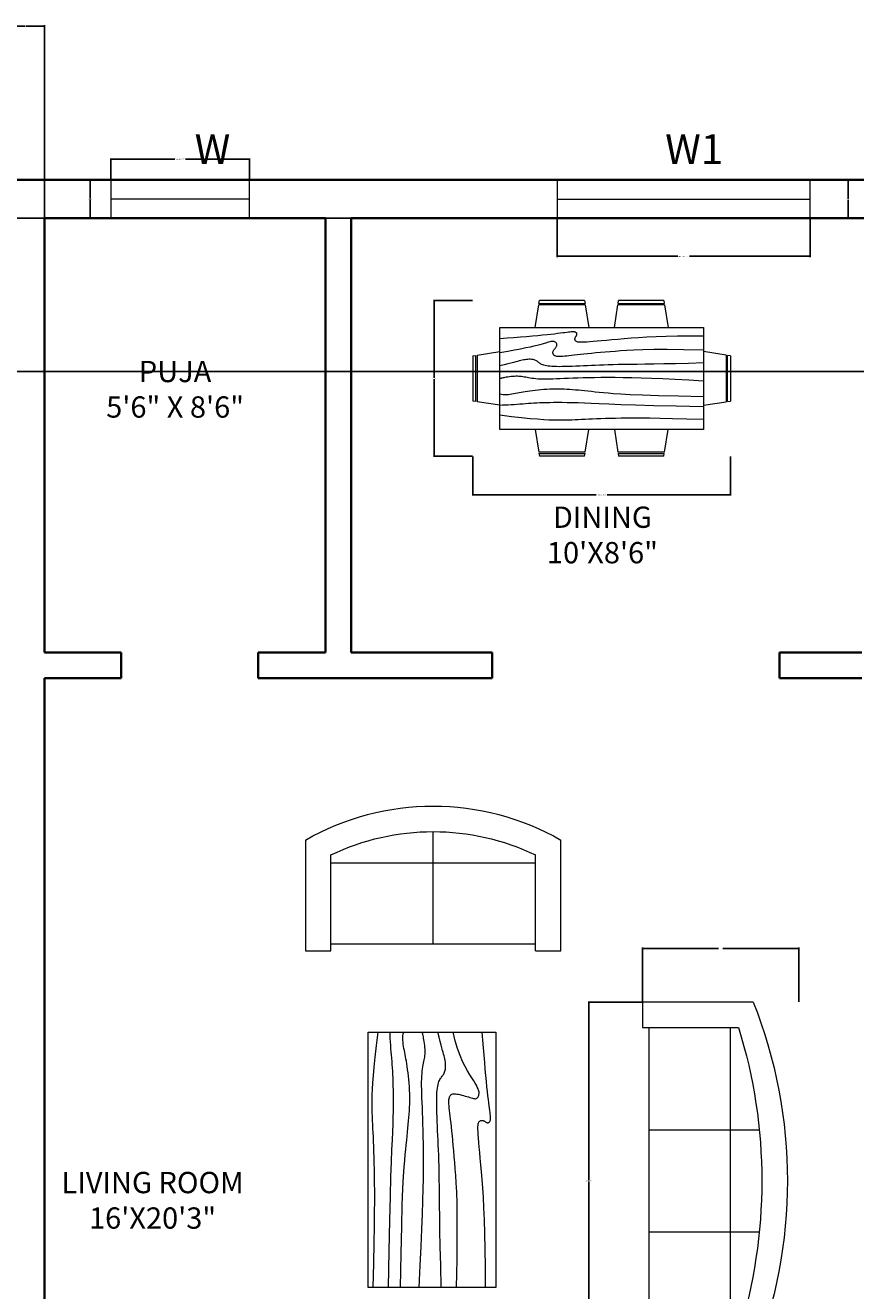
# Model space of a CAD drawing. Units: inches. Extents: x 1939 to 2674, y 558 to 1170.
# Tile 5 of 6: x 2307 to 2502, y 873 to 1170. Entities that reach past the tile are written whole.
import ezdxf

# ---------------------------------------------------------------- set-up
doc = ezdxf.new("R2010")
doc.units = ezdxf.units.IN
for name, color, linetype, lineweight in [('A-ANNO-DIMS', 2, 'Continuous', 18), ('A-ANNO-TEXT', 7, 'Continuous', 18), ('A-AREA-IDEN', 7, 'Continuous', 18), ('A-FURN', 8, 'Continuous', 13), ('A-GLAZ', 4, 'Continuous', 18), ('A-WALL', 7, 'Continuous', 35)]:
    doc.layers.add(name, color=color, linetype=linetype, lineweight=lineweight)
doc.styles.get("Standard").update_dxf_attribs({"font": 'arial.ttf'})
doc.dimstyles.get("Standard").update_dxf_attribs({"dimtxt": 0.18, "dimasz": 0.18, "dimexe": 0.18, "dimexo": 0.0625, "dimgap": 0.09, "dimtad": 0, "dimtih": 1, "dimtoh": 1, "dimdec": 4, "dimzin": 0, "dimdsep": 46, "dimtxsty": 'Standard', "dimcen": 0.09, "dimadec": 0, "dimazin": 0, "dimtfac": 1, "dimtdec": 4, "dimtofl": 0, "dimtmove": 0, "dimatfit": 3, "dimfxl": 1, "dimtolj": 1, "dimtzin": 0, "dimarcsym": 0})

# ---------------------------------------------------------------- blocks, each defined once
blk = doc.blocks.new('Dining Set - 36 x 72 in.')
for p, q in [((-22, 27.5), (-22.1562, 26.50042)), ((-22, 27.5), (-6, 27.5)), ((-5.8437, 26.49966), (-6, 27.5)), ((6, 27.5), (5.8438, 26.50042)), ((6, 27.5), (22, 27.5)), ((22.1563, 26.49966), (22, 27.5)), ((-22.2343, 26.00059), (-23.4847, 17.99762)), ((-22.2304, 26), (-5.7608, 26)), ((-5.8416, 26.5), (-22.1534, 26.5)), ((-4.5152, 17.99762), (-5.7655, 25.99926)), ((5.7657, 26.00059), (4.5153, 17.99762)), ((5.7696, 26), (22.2392, 26)), ((22.1584, 26.5), (5.8466, 26.5)), ((23.4848, 17.99762), (22.2345, 25.99926)), ((36, 18), (-36, 18)), ((-36, 18), (-36, -18)), ((36, -18), (36, 18)), ((-44.0006, 8.23428), (-35.9976, 9.48474)), ((44.0006, 8.23428), (35.9976, 9.48474)), ((-45.5, 8), (-44.5004, 8.15617)), ((-45.5, 8), (-45.5, -8)), ((-44.5, -8.15843), (-44.5, 8.15338)), ((-44, 8.23041), (-44, -8.23915)), ((44, 8.23041), (44, -8.23915)), ((44.5, -8.15843), (44.5, 8.15338)), ((45.5, 8), (44.5005, 8.15617)), ((45.5, 8), (45.5, -8)), ((-44.4997, -8.15631), (-45.5, -8)), ((-35.9976, -9.48476), (-43.9993, -8.2345)), ((35.9976, -9.48476), (43.9993, -8.2345)), ((44.4997, -8.15631), (45.5, -8)), ((-36, -18), (36, -18)), ((-22.2343, -26.0006), (-23.4847, -17.99762)), ((-4.5152, -17.99762), (-5.7655, -25.99928)), ((5.7657, -26.0006), (4.5153, -17.99762)), ((23.4848, -17.99762), (22.2345, -25.99928)), ((-22.2304, -26), (-5.7608, -26)), ((-22, -27.5), (-22.1562, -26.50044)), ((-5.8416, -26.5), (-22.1534, -26.5)), ((-5.8437, -26.49967), (-6, -27.5)), ((5.7696, -26), (22.2392, -26)), ((6, -27.5), (5.8438, -26.50044)), ((22.1584, -26.5), (5.8466, -26.5)), ((22.1563, -26.49967), (22, -27.5)), ((-22, -27.5), (-6, -27.5)), ((6, -27.5), (22, -27.5))]:
    blk.add_line(p, q)
for points in [[(-36, 15), (-31.1772, 14.97754), (-26.8079, 14.91406), (-22.8538, 14.81543), (-19.276, 14.6875), (-16.0362, 14.53613), (-13.0957, 14.36718), (-10.4159, 14.18652), (-7.9583, 14), (-5.6904, 13.81315), (-3.6035, 13.63021), (-1.6954, 13.45508), (0.0365, 13.29166), (1.5945, 13.14388), (2.9811, 13.01562), (4.1988, 12.9108), (5.25, 12.83333), (6.1393, 12.78613), (6.8802, 12.76823), (7.4883, 12.77767), (7.9792, 12.8125), (8.3685, 12.87077), (8.6719, 12.95052), (8.9049, 13.0498), (9.0833, 13.16666), (9.2205, 13.29899), (9.3216, 13.44401), (9.3895, 13.59879), (9.4271, 13.76041), (9.4373, 13.92594), (9.4232, 14.09245), (9.3875, 14.257), (9.3333, 14.41666), (9.2638, 14.56917), (9.1836, 14.71484), (9.0975, 14.85465), (9.0104, 14.98958), (8.9272, 15.1206), (8.8529, 15.2487), (8.7922, 15.37483), (8.75, 15.5), (8.7305, 15.62467), (8.7344, 15.74739), (8.7617, 15.86621), (8.8125, 15.97916), (8.8867, 16.08431), (8.9844, 16.17968), (9.1055, 16.26334), (9.25, 16.33333), (9.4189, 16.38802), (9.6172, 16.42708), (9.8506, 16.45052), (10.125, 16.45833), (10.4463, 16.45052), (10.8203, 16.42708), (11.2529, 16.38802), (11.75, 16.33333), (12.3184, 16.26318), (12.9694, 16.17838), (13.7151, 16.07991), (14.5677, 15.96875), (15.5395, 15.84586), (16.6426, 15.71224), (17.8893, 15.56884), (19.2917, 15.41666), (20.859, 15.25667), (22.5879, 15.08984), (24.4721, 14.91715), (26.5052, 14.73958), (28.6809, 14.5581), (30.9929, 14.3737), (33.4347, 14.18733), (36, 14)], [(-36, 10), (-28.9766, 10.14274), (-23.1725, 10.20442), (-18.4241, 10.19775), (-14.5677, 10.13541), (-11.4399, 10.03011), (-8.877, 9.89453), (-6.7154, 9.74137), (-4.7917, 9.58333), (-2.9698, 9.43082), (-1.2246, 9.28515), (0.4415, 9.14534), (2.026, 9.01041), (3.5266, 8.87939), (4.9408, 8.7513), (6.266, 8.62516), (7.5, 8.5), (8.6411, 8.37549), (9.6914, 8.2539), (10.6538, 8.13818), (11.5312, 8.03125), (12.3267, 7.93603), (13.043, 7.85547), (13.6831, 7.79248), (14.25, 7.75), (14.7471, 7.7303), (15.1797, 7.73307), (15.5537, 7.75732), (15.875, 7.80208), (16.1494, 7.86637), (16.3828, 7.94922), (16.5811, 8.04964), (16.75, 8.16666), (16.8944, 8.29915), (17.0143, 8.44531), (17.1089, 8.60319), (17.1771, 8.77083), (17.218, 8.94629), (17.2305, 9.1276), (17.2137, 9.31282), (17.1667, 9.5), (17.0895, 9.6875), (16.987, 9.875), (16.8649, 10.0625), (16.7292, 10.25), (16.5856, 10.4375), (16.4401, 10.625), (16.2985, 10.8125), (16.1667, 11), (16.05, 11.18733), (15.9518, 11.3737), (15.8752, 11.5581), (15.8229, 11.73958), (15.798, 11.91715), (15.8034, 12.08984), (15.842, 12.25667), (15.9167, 12.41666), (16.0295, 12.56836), (16.1784, 12.70833), (16.3605, 12.83268), (16.5729, 12.9375), (16.8127, 13.01888), (17.0768, 13.07291), (17.3625, 13.0957), (17.6667, 13.08333), (17.9894, 13.03312), (18.3418, 12.94726), (18.7382, 12.82918), (19.1927, 12.68229), (19.7195, 12.51001), (20.3327, 12.31575), (21.0465, 12.10294), (21.875, 11.875), (22.8357, 11.63354), (23.959, 11.37304), (25.2786, 11.08618), (26.8282, 10.76562), (28.6414, 10.40405), (30.752, 9.99414), (33.1936, 9.52856), (36, 9)], [(-36, 5.5), (-30.7157, 5.3348), (-26.069, 5.20963), (-21.9946, 5.11767), (-18.4271, 5.05208), (-15.3009, 5.00602), (-12.5508, 4.97265), (-10.1112, 4.94515), (-7.9167, 4.91666), (-5.909, 4.88167), (-4.0586, 4.83984), (-2.3429, 4.79215), (-0.7396, 4.73958), (0.7739, 4.6831), (2.22, 4.6237), (3.6213, 4.56233), (5, 4.5), (6.373, 4.43782), (7.7344, 4.3776), (9.0723, 4.32129), (10.375, 4.27083), (11.6309, 4.22819), (12.8281, 4.19531), (13.9551, 4.17415), (15, 4.16666), (15.954, 4.17448), (16.819, 4.19791), (17.6001, 4.23698), (18.3021, 4.29166), (18.9299, 4.36198), (19.4883, 4.44791), (19.9823, 4.54948), (20.4167, 4.66666), (20.7969, 4.79899), (21.1302, 4.94401), (21.4245, 5.09879), (21.6875, 5.26041), (21.9271, 5.42594), (22.1511, 5.59245), (22.3672, 5.757), (22.5834, 5.91666), (22.8065, 6.06868), (23.0404, 6.21093), (23.2879, 6.34147), (23.5521, 6.45833), (23.8358, 6.55957), (24.142, 6.64323), (24.4735, 6.70735), (24.8334, 6.75), (25.2235, 6.76969), (25.642, 6.76692), (26.0858, 6.74267), (26.5521, 6.69791), (27.0379, 6.63362), (27.5404, 6.55078), (28.0565, 6.45036), (28.5834, 6.33333), (29.1242, 6.19987), (29.7071, 6.04687), (30.3661, 5.87044), (31.1354, 5.66666), (32.0493, 5.43164), (33.142, 5.16146), (34.4475, 4.85221), (36, 4.5)], [(-36, -1), (-30.7915, -0.6591), (-26.0195, -0.38216), (-21.6519, -0.16284), (-17.6563, 0.00521), (-14.0005, 0.12833), (-10.6523, 0.21289), (-7.5796, 0.26522), (-4.75, 0.29166), (-2.134, 0.29793), (0.2878, 0.28711), (2.5317, 0.26163), (4.6146, 0.22396), (6.5529, 0.17651), (8.3633, 0.12174), (10.0623, 0.06209), (11.6667, 0), (13.1899, -0.06201), (14.6341, -0.1211), (15.9982, -0.17432), (17.2813, -0.21875), (18.4823, -0.25147), (19.6003, -0.26953), (20.6343, -0.27002), (21.5834, -0.25), (22.4481, -0.20768), (23.2357, -0.14584), (23.9549, -0.06836), (24.6146, 0.02083), (25.2235, 0.11784), (25.7904, 0.21875), (26.3241, 0.31966), (26.8334, 0.41666), (27.3265, 0.50618), (27.8099, 0.58593), (28.2894, 0.65397), (28.7709, 0.70833), (29.2601, 0.74707), (29.763, 0.76823), (30.2855, 0.76985), (30.8334, 0.75), (31.4088, 0.70784), (31.9994, 0.64713), (32.589, 0.57275), (33.1615, 0.48958), (33.7008, 0.4025), (34.1908, 0.3164), (34.6153, 0.23616), (34.9584, 0.16666), (35.2099, 0.11165), (35.3848, 0.07031), (35.504, 0.04069), (35.5886, 0.02083), (35.6594, 0.00879), (35.7377, 0.0026), (35.8442, 0.00032), (36, 0)], [(-36, -6.5), (-27.1843, -6.31267), (-20.084, -6.1263), (-14.469, -5.9419), (-10.1094, -5.76042), (-6.7752, -5.58285), (-4.2363, -5.41016), (-2.2629, -5.24333), (-0.625, -5.08334), (0.8708, -4.93099), (2.2715, -4.78646), (3.5872, -4.64974), (4.8281, -4.52084), (6.0046, -4.39974), (7.127, -4.28646), (8.2053, -4.18099), (9.25, -4.08334), (10.2705, -3.99382), (11.2734, -3.91407), (12.2647, -3.84603), (13.25, -3.79167), (14.2354, -3.75293), (15.2266, -3.73177), (16.2295, -3.73015), (17.25, -3.75), (18.2912, -3.79248), (19.3451, -3.85547), (20.4009, -3.93604), (21.4479, -4.03125), (22.4754, -4.13819), (23.4727, -4.25391), (24.4289, -4.37549), (25.3334, -4.5), (26.1785, -4.62492), (26.9694, -4.74935), (27.7145, -4.87281), (28.4219, -4.99479), (29.1, -5.11483), (29.7572, -5.23242), (30.4016, -5.34709), (31.0417, -5.45834), (31.6837, -5.56437), (32.3262, -5.65821), (32.9658, -5.73153), (33.599, -5.77604), (34.2224, -5.78345), (34.8327, -5.74545), (35.4264, -5.65373), (36, -5.5)], [(-36, -10), (-26.4022, -9.81299), (-18.4675, -9.62891), (-11.9839, -9.45069), (-6.7396, -9.28125), (-2.5226, -9.12354), (0.8789, -8.98047), (3.6769, -8.85498), (6.0833, -8.75), (8.2767, -8.66765), (10.3021, -8.60677), (12.1712, -8.56543), (13.8958, -8.54167), (15.4876, -8.53353), (16.9583, -8.53907), (18.3197, -8.55632), (19.5834, -8.58334), (20.7616, -8.61841), (21.8685, -8.66081), (22.9188, -8.71004), (23.9271, -8.76563), (24.9081, -8.82707), (25.8763, -8.89388), (26.8465, -8.96558), (27.8334, -9.04167), (28.8474, -9.12118), (29.8828, -9.20117), (30.93, -9.27824), (31.9792, -9.34896), (33.0205, -9.40991), (34.0443, -9.45768), (35.0407, -9.48885), (36, -9.5)], [(-36, -14.5), (-30.0881, -14.33513), (-25.0332, -14.21224), (-20.7312, -14.12647), (-17.0781, -14.07292), (-13.97, -14.04671), (-11.3027, -14.04297), (-8.9724, -14.05681), (-6.875, -14.08334), (-4.9224, -14.11833), (-3.0905, -14.16016), (-1.3709, -14.20785), (0.2448, -14.26042), (1.7647, -14.3169), (3.1973, -14.3763), (4.5507, -14.43767), (5.8333, -14.5), (7.0554, -14.5621), (8.235, -14.62175), (9.3922, -14.67652), (10.5469, -14.72396), (11.7192, -14.76164), (12.929, -14.78711), (14.1965, -14.79794), (15.5417, -14.79167), (16.9933, -14.76424), (18.6152, -14.70508), (20.4804, -14.60197), (22.6615, -14.44271), (25.2312, -14.21509), (28.2624, -13.9069), (31.8277, -13.50594), (36, -13)]]:
    blk.add_lwpolyline(points)
blk = doc.blocks.new('Sofa - Roundback 7 ft.')
for p, q in [((-12.00002, -32.4421), (-12.00003, -6.5971)), ((11.99997, -32.4421), (11.99998, -6.5971)), ((-36.000027, -34), (-36.000027, -11.4696)), ((35.99998, -34), (35.99998, -11.4696)), ((-35.999844, -13.3819), (35.9998, -13.3819)), ((-36.000027, -32.4421), (35.99998, -32.4421))]:
    blk.add_line(p, q)
for points in [[(-36.000027, -34), (-42.000027, -34), (-42.000027, -8)], [(41.99998, -8), (41.99998, -34), (35.99998, -34)]]:
    blk.add_lwpolyline(points)
for centre, radius, start, end in [((0, -114.25), 114.25, 68.43141, 111.5686), ((-0.00001, -127.1968), 121.1968, 72.72033, 107.2797)]:
    blk.add_arc(centre, radius, start, end)
blk = doc.blocks.new('Sofa - Roundback Loveseat 5 ft.')
for p, q in [((0, -32.44198), (0, -5.99998)), ((-24, -33.99998), (-24, -11.46958)), ((24.00004, -33.99998), (24.00004, -11.46958)), ((-23.9998, -13.38178), (23.99986, -13.38178)), ((-24, -32.44198), (24.00004, -32.44198))]:
    blk.add_line(p, q)
for points in [[(-24, -33.99998), (-30, -33.99998), (-30, -7.99998)], [(30.00004, -7.99998), (30.00004, -33.99998), (24.00004, -33.99998)]]:
    blk.add_lwpolyline(points)
for centre, radius, start, end in [((0, -60.24998), 60.24998, 60.13715, 119.8628), ((0, -61.38438), 55.38444, 64.32083, 115.6792)]:
    blk.add_arc(centre, radius, start, end)
blk = doc.blocks.new('Table - Rectangular Woodgrain 60 x 30 in.')
for p, q in [((0, 0), (0, -30)), ((60, 0), (0, 0)), ((60, -30), (60, 0)), ((0, -30), (60, -30))]:
    blk.add_line(p, q)
for points in [[(0, -2.4), (4.8155, -2.418), (9.0302, -2.4688), (12.709, -2.5477), (15.9167, -2.65), (18.7181, -2.7711), (21.1781, -2.9063), (23.3616, -3.0508), (25.3333, -3.2), (27.1477, -3.3495), (28.8172, -3.4958), (30.3437, -3.636), (31.7291, -3.7667), (32.9756, -3.8849), (34.0849, -3.9875), (35.059, -4.0714), (35.9, -4.1334), (36.6114, -4.1711), (37.2041, -4.1854), (37.6906, -4.1779), (38.0833, -4.15), (38.3948, -4.1034), (38.6375, -4.0396), (38.8239, -3.9602), (38.9666, -3.8667), (39.0764, -3.7608), (39.1573, -3.6448), (39.2116, -3.521), (39.2416, -3.3917), (39.2498, -3.2593), (39.2385, -3.1261), (39.21, -2.9944), (39.1666, -2.8667), (39.111, -2.7447), (39.0468, -2.6281), (38.978, -2.5163), (38.9083, -2.4083), (38.8418, -2.3035), (38.7823, -2.201), (38.7337, -2.1001), (38.7, -2), (38.6844, -1.9003), (38.6875, -1.8021), (38.7094, -1.707), (38.75, -1.6167), (38.8094, -1.5326), (38.8875, -1.4563), (38.9844, -1.3893), (39.1, -1.3333), (39.2351, -1.2896), (39.3937, -1.2583), (39.5804, -1.2396), (39.8, -1.2333), (40.057, -1.2396), (40.3562, -1.2583), (40.7023, -1.2896), (41.1, -1.3333), (41.5547, -1.3895), (42.0755, -1.4573), (42.6721, -1.5361), (43.3542, -1.625), (44.1316, -1.7233), (45.014, -1.8302), (46.0114, -1.9449), (47.1333, -2.0667), (48.3862, -2.1947), (49.7625, -2.3281), (51.2513, -2.4663), (52.8416, -2.6083), (54.5226, -2.7535), (56.2833, -2.9011), (58.1127, -3.0501), (60, -3.2)], [(0, -9.2), (6.5759, -9.0858), (11.9385, -9.0365), (16.2527, -9.0418), (19.6833, -9.0917), (22.3952, -9.1759), (24.5531, -9.2844), (26.322, -9.4069), (27.8666, -9.5333), (29.3241, -9.6553), (30.7203, -9.7719), (32.0532, -9.8837), (33.3208, -9.9917), (34.5213, -10.0965), (35.6526, -10.199), (36.7128, -10.2999), (37.7, -10.4), (38.6129, -10.4996), (39.4531, -10.5969), (40.223, -10.6895), (40.925, -10.775), (41.5613, -10.8512), (42.1344, -10.9156), (42.6465, -10.966), (43.1, -11), (43.4976, -11.0158), (43.8437, -11.0136), (44.143, -10.9942), (44.4, -10.9583), (44.6195, -10.9069), (44.8062, -10.8406), (44.9648, -10.7603), (45.1, -10.6667), (45.2155, -10.5598), (45.3114, -10.4365), (45.3871, -10.2929), (45.4416, -10.125), (45.4743, -9.929), (45.4844, -9.7011), (45.4709, -9.4371), (45.4333, -9.1333), (45.3716, -8.7883), (45.2896, -8.4104), (45.1919, -8.0107), (45.0833, -7.6), (44.9685, -7.1893), (44.8521, -6.7896), (44.7388, -6.4117), (44.6333, -6.0667), (44.54, -5.7628), (44.4614, -5.4979), (44.4001, -5.2675), (44.3583, -5.0667), (44.3384, -4.8909), (44.3427, -4.7354), (44.3736, -4.5956), (44.4333, -4.4667), (44.5236, -4.3453), (44.6427, -4.2333), (44.7884, -4.1339), (44.9583, -4.05), (45.1501, -3.9849), (45.3614, -3.9417), (45.59, -3.9234), (45.8333, -3.9333), (46.0915, -3.9749), (46.3734, -4.0531), (46.6906, -4.1736), (47.0542, -4.3417), (47.4756, -4.5629), (47.9661, -4.8427), (48.5372, -5.1866), (49.2, -5.6), (49.9676, -6.0844), (50.8594, -6.625), (51.8965, -7.2031), (53.1, -7.8), (54.491, -8.3969), (56.0906, -8.975), (57.9199, -9.5156), (60, -10)], [(0, -12.8), (5.1847, -12.9322), (9.6213, -13.0323), (13.3963, -13.1059), (16.5958, -13.1583), (19.3063, -13.1952), (21.614, -13.2219), (23.6054, -13.2439), (25.3666, -13.2667), (26.9728, -13.2947), (28.4531, -13.3281), (29.8256, -13.3663), (31.1083, -13.4083), (32.3191, -13.4535), (33.476, -13.501), (34.597, -13.5501), (35.7, -13.6), (36.7984, -13.6497), (37.8875, -13.6979), (38.9578, -13.743), (40, -13.7833), (41.0047, -13.8174), (41.9625, -13.8438), (42.864, -13.8607), (43.7, -13.8667), (44.4631, -13.8604), (45.1552, -13.8417), (45.7801, -13.8104), (46.3416, -13.7667), (46.8439, -13.7104), (47.2906, -13.6417), (47.6858, -13.5604), (48.0333, -13.4667), (48.3375, -13.3608), (48.6042, -13.2448), (48.8396, -13.121), (49.05, -12.9917), (49.2417, -12.8593), (49.4208, -12.7261), (49.5937, -12.5944), (49.7667, -12.4667), (49.9452, -12.3451), (50.1323, -12.2313), (50.3303, -12.1268), (50.5416, -12.0333), (50.7686, -11.9524), (51.0135, -11.8854), (51.2788, -11.8341), (51.5666, -11.8), (51.8785, -11.7843), (52.2116, -11.7865), (52.562, -11.8059), (52.926, -11.8417), (53.2998, -11.8931), (53.6795, -11.9594), (54.0614, -12.0397), (54.4416, -12.1333), (54.8223, -12.2401), (55.2293, -12.3625), (55.6942, -12.5037), (56.2489, -12.6667), (56.9251, -12.8547), (57.7545, -13.0708), (58.7689, -13.3182), (60, -13.6)], [(0, -18), (5.124, -17.7273), (9.6609, -17.5057), (13.6705, -17.3303), (17.2125, -17.1958), (20.3467, -17.0973), (23.1328, -17.0297), (25.6307, -16.9878), (27.9, -16.9667), (29.9928, -16.9617), (31.9302, -16.9703), (33.7254, -16.9907), (35.3917, -17.0208), (36.9423, -17.0588), (38.3906, -17.1026), (39.7499, -17.1503), (41.0333, -17.2), (42.2519, -17.2496), (43.4073, -17.2969), (44.4986, -17.3395), (45.525, -17.375), (46.4858, -17.4012), (47.3802, -17.4156), (48.2074, -17.416), (48.9667, -17.4), (49.6583, -17.3662), (50.2872, -17.3167), (50.8595, -17.2547), (51.3812, -17.1833), (51.8584, -17.1057), (52.2971, -17.025), (52.7034, -16.9443), (53.0833, -16.8667), (53.443, -16.7951), (53.789, -16.7313), (54.128, -16.6768), (54.4666, -16.6334), (54.8115, -16.6024), (55.1693, -16.5854), (55.5465, -16.5841), (55.95, -16.6), (56.3828, -16.6337), (56.8346, -16.6823), (57.2915, -16.7418), (57.7396, -16.8084), (58.165, -16.878), (58.5539, -16.9469), (58.8924, -17.0111), (59.1666, -17.0667), (59.3679, -17.1107), (59.5078, -17.1438), (59.6032, -17.1675), (59.6708, -17.1833), (59.7275, -17.193), (59.7901, -17.1979), (59.8753, -17.1998), (60, -17.2)], [(0, -22.4), (8.0098, -22.2501), (14.4094, -22.1011), (19.4168, -21.9535), (23.25, -21.8083), (26.1269, -21.6663), (28.2656, -21.5281), (29.884, -21.3947), (31.2, -21.2667), (32.3967, -21.1448), (33.5172, -21.0292), (34.5697, -20.9198), (35.5625, -20.8167), (36.5037, -20.7198), (37.4015, -20.6292), (38.2642, -20.5448), (39.1, -20.4667), (39.9164, -20.3951), (40.7187, -20.3313), (41.5117, -20.2768), (42.3, -20.2333), (43.0883, -20.2024), (43.8812, -20.1854), (44.6836, -20.1841), (45.5, -20.2), (46.3328, -20.234), (47.1747, -20.2844), (48.0163, -20.3488), (48.8479, -20.425), (49.66, -20.5106), (50.4429, -20.6031), (51.1872, -20.7004), (51.8833, -20.8), (52.5246, -20.8999), (53.1166, -20.9995), (53.6681, -21.0983), (54.1875, -21.1958), (54.6834, -21.2919), (55.1646, -21.3859), (55.6394, -21.4777), (56.1167, -21.5667), (56.6028, -21.6515), (57.0961, -21.7266), (57.5929, -21.7852), (58.0896, -21.8208), (58.5823, -21.8268), (59.0674, -21.7964), (59.5412, -21.723), (60, -21.6)], [(0, -25.2), (8.6355, -25.0504), (15.7026, -24.9031), (21.4049, -24.7606), (25.9458, -24.625), (29.529, -24.4988), (32.3578, -24.3844), (34.6359, -24.284), (36.5667, -24.2), (38.3213, -24.1341), (39.9417, -24.0854), (41.437, -24.0523), (42.8167, -24.0333), (44.0901, -24.0268), (45.2667, -24.0313), (46.3557, -24.0451), (47.3667, -24.0667), (48.309, -24.0947), (49.1928, -24.1287), (50.0284, -24.168), (50.826, -24.2125), (51.5959, -24.2617), (52.3483, -24.3151), (53.0935, -24.3725), (53.8417, -24.4334), (54.6009, -24.497), (55.3699, -24.561), (56.1454, -24.6226), (56.9239, -24.6792), (57.7021, -24.7279), (58.4764, -24.7662), (59.2435, -24.7911), (60, -24.8)], [(0, -28.8), (5.6867, -28.6681), (10.45, -28.5698), (14.407, -28.5012), (17.675, -28.4584), (20.3711, -28.4374), (22.6125, -28.4344), (24.5164, -28.4455), (26.2, -28.4667), (27.762, -28.4947), (29.2276, -28.5281), (30.6033, -28.5663), (31.8958, -28.6084), (33.1118, -28.6535), (34.2578, -28.7011), (35.3405, -28.7501), (36.3666, -28.8), (37.3443, -28.8497), (38.288, -28.8974), (39.2137, -28.9412), (40.1375, -28.9792), (41.0753, -29.0093), (42.0432, -29.0297), (43.0572, -29.0384), (44.1333, -29.0333), (45.2936, -29.0114), (46.5843, -28.9641), (48.0579, -28.8816), (49.7666, -28.7542), (51.7629, -28.5721), (54.0989, -28.3255), (56.8272, -28.0048), (60, -27.6)]]:
    blk.add_lwpolyline(points)
blk = doc.blocks.new('WIN-PUJA')
for p, q in [((0, 9), (0, 0)), ((32.53, 0), (32.53, 9)), ((0, 4.5), (32.53, 4.5))]:
    blk.add_line(p, q)
blk = doc.blocks.new('WIN-DINING')
for p, q in [((0, 9), (0, 0)), ((59.38, 0), (59.38, 9)), ((0, 4.5), (59.38, 4.5))]:
    blk.add_line(p, q)
blk = doc.blocks.new('*D24')
at = {"layer": 'A-ANNO-DIMS', "color": 0, "lineweight": -2, "transparency": 16777216}
for p, q in [((2411.67, 1069.16), (2411.67, 1059.97)), ((2472.14, 1069.16), (2472.14, 1059.97)), ((2411.85, 1060.15), (2440.62, 1060.15)), ((2471.96, 1060.15), (2443.18, 1060.15))]:
    blk.add_line(p, q, dxfattribs=at)
at = {"layer": 'A-ANNO-DIMS', "color": 0, "transparency": 16777216}
for points in [[(2411.85, 1060.18), (2411.85, 1060.12), (2411.67, 1060.15)], [(2471.96, 1060.18), (2471.96, 1060.12), (2472.14, 1060.15)]]:
    blk.add_solid(points, dxfattribs=at)
at = {"layer": 'Defpoints', "color": 0, "transparency": 16777216}
for p in [(2411.67, 1069.22), (2472.14, 1069.22), (2411.67, 1060.15)]:
    blk.add_point(p, dxfattribs=at)
at = {"layer": 'A-ANNO-DIMS', "color": 0, "transparency": 16777216, "insert": (2441.9, 1060.15), "char_height": 0.18, "attachment_point": 5}
blk.add_mtext('\\A1;DINING SET 60 TYP.', dxfattribs=at)
blk = doc.blocks.new('*D25')
at = {"layer": 'A-ANNO-DIMS', "color": 0, "lineweight": -2, "transparency": 16777216}
for p, q in [((2411.61, 1105.77), (2402.42, 1105.77)), ((2402.6, 1105.59), (2402.6, 1087.68)), ((2402.6, 1069.4), (2402.6, 1087.32)), ((2411.61, 1069.22), (2402.42, 1069.22))]:
    blk.add_line(p, q, dxfattribs=at)
at = {"layer": 'A-ANNO-DIMS', "color": 0, "transparency": 16777216}
for points in [[(2402.57, 1105.59), (2402.63, 1105.59), (2402.6, 1105.77)], [(2402.57, 1069.4), (2402.63, 1069.4), (2402.6, 1069.22)]]:
    blk.add_solid(points, dxfattribs=at)
at = {"layer": 'Defpoints', "color": 0, "transparency": 16777216}
for p in [(2402.6, 1105.77), (2411.67, 1105.77), (2411.67, 1069.22)]:
    blk.add_point(p, dxfattribs=at)
at = {"layer": 'A-ANNO-DIMS', "color": 0, "transparency": 16777216, "insert": (2402.6, 1087.5), "char_height": 0.18, "attachment_point": 5}
blk.add_mtext('\\A1;37 TYP.', dxfattribs=at)
blk = doc.blocks.new('*D26')
at = {"layer": 'A-ANNO-DIMS', "color": 0, "lineweight": -2, "transparency": 16777216}
for p, q in [((2451.46, 941.04), (2438.74, 941.04)), ((2438.92, 940.86), (2438.92, 899.23)), ((2438.92, 857.22), (2438.92, 898.86)), ((2451.46, 857.04), (2438.74, 857.04))]:
    blk.add_line(p, q, dxfattribs=at)
at = {"layer": 'A-ANNO-DIMS', "color": 0, "transparency": 16777216}
for points in [[(2438.89, 940.86), (2438.95, 940.86), (2438.92, 941.04)], [(2438.89, 857.22), (2438.95, 857.22), (2438.92, 857.04)]]:
    blk.add_solid(points, dxfattribs=at)
at = {"layer": 'Defpoints', "color": 0, "transparency": 16777216}
for p in [(2438.92, 941.04), (2451.52, 941.04), (2451.52, 857.04)]:
    blk.add_point(p, dxfattribs=at)
at = {"layer": 'A-ANNO-DIMS', "color": 0, "transparency": 16777216, "insert": (2438.92, 899.04), "char_height": 0.18, "attachment_point": 5}
blk.add_mtext('\\A1;SOFA 84 TYP.', dxfattribs=at)
blk = doc.blocks.new('*D27')
at = {"layer": 'A-ANNO-DIMS', "color": 0, "lineweight": -2, "transparency": 16777216}
for p, q in [((2451.52, 941.11), (2451.52, 953.82)), ((2451.7, 953.64), (2469.33, 953.64)), ((2488.01, 953.64), (2470.39, 953.64)), ((2488.19, 941.11), (2488.19, 953.82))]:
    blk.add_line(p, q, dxfattribs=at)
at = {"layer": 'A-ANNO-DIMS', "color": 0, "transparency": 16777216}
for points in [[(2451.7, 953.67), (2451.7, 953.61), (2451.52, 953.64)], [(2488.01, 953.67), (2488.01, 953.61), (2488.19, 953.64)]]:
    blk.add_solid(points, dxfattribs=at)
at = {"layer": 'Defpoints', "color": 0, "transparency": 16777216}
for p in [(2488.19, 953.64), (2451.52, 941.04), (2488.19, 941.04)]:
    blk.add_point(p, dxfattribs=at)
at = {"layer": 'A-ANNO-DIMS', "color": 0, "transparency": 16777216, "insert": (2469.86, 953.64), "char_height": 0.18, "attachment_point": 5}
blk.add_mtext('\\A1;37 TYP.', dxfattribs=at)
blk = doc.blocks.new('*D36')
at = {"layer": 'A-ANNO-DIMS', "color": 0, "lineweight": -2, "transparency": 16777216}
for p, q in [((2326.67, 1134.17), (2326.67, 1139.17)), ((2326.85, 1138.99), (2341.69, 1138.99)), ((2359.02, 1138.99), (2344.18, 1138.99)), ((2359.2, 1134.17), (2359.2, 1139.17))]:
    blk.add_line(p, q, dxfattribs=at)
at = {"layer": 'A-ANNO-DIMS', "color": 0, "transparency": 16777216}
for points in [[(2326.85, 1139.02), (2326.85, 1138.96), (2326.67, 1138.99)], [(2359.02, 1139.02), (2359.02, 1138.96), (2359.2, 1138.99)]]:
    blk.add_solid(points, dxfattribs=at)
at = {"layer": 'Defpoints', "color": 0, "transparency": 16777216}
for p in [(2326.67, 1138.99), (2326.67, 1134.11), (2359.2, 1134.11)]:
    blk.add_point(p, dxfattribs=at)
at = {"layer": 'A-ANNO-DIMS', "color": 0, "transparency": 16777216, "insert": (2342.93, 1138.99), "char_height": 0.18, "attachment_point": 5}
blk.add_mtext('\\A1;PUJA WDW 33 TYP.', dxfattribs=at)
blk = doc.blocks.new('*D37')
at = {"layer": 'A-ANNO-DIMS', "color": 0, "lineweight": -2, "transparency": 16777216}
for p, q in [((2326.61, 1134.11), (2321.61, 1134.11)), ((2321.79, 1133.93), (2321.79, 1129.79)), ((2321.79, 1125.29), (2321.79, 1129.43)), ((2326.61, 1125.11), (2321.61, 1125.11))]:
    blk.add_line(p, q, dxfattribs=at)
at = {"layer": 'A-ANNO-DIMS', "color": 0, "transparency": 16777216}
for points in [[(2321.76, 1133.93), (2321.82, 1133.93), (2321.79, 1134.11)], [(2321.76, 1125.29), (2321.82, 1125.29), (2321.79, 1125.11)]]:
    blk.add_solid(points, dxfattribs=at)
at = {"layer": 'Defpoints', "color": 0, "transparency": 16777216}
for p in [(2326.67, 1134.11), (2321.79, 1125.11), (2326.67, 1125.11)]:
    blk.add_point(p, dxfattribs=at)
at = {"layer": 'A-ANNO-DIMS', "color": 0, "transparency": 16777216, "insert": (2321.79, 1129.61), "char_height": 0.18, "attachment_point": 5}
blk.add_mtext('\\A1;9 TYP.', dxfattribs=at)
blk = doc.blocks.new('*D38')
at = {"layer": 'A-ANNO-DIMS', "color": 0, "lineweight": -2, "transparency": 16777216}
for p, q in [((2431.49, 1125.05), (2431.49, 1116.02)), ((2490.87, 1125.05), (2490.87, 1116.02)), ((2431.67, 1116.2), (2459.82, 1116.2)), ((2490.69, 1116.2), (2462.54, 1116.2))]:
    blk.add_line(p, q, dxfattribs=at)
at = {"layer": 'A-ANNO-DIMS', "color": 0, "transparency": 16777216}
for points in [[(2431.67, 1116.23), (2431.67, 1116.17), (2431.49, 1116.2)], [(2490.69, 1116.23), (2490.69, 1116.17), (2490.87, 1116.2)]]:
    blk.add_solid(points, dxfattribs=at)
at = {"layer": 'Defpoints', "color": 0, "transparency": 16777216}
for p in [(2431.49, 1125.11), (2490.87, 1125.11), (2490.87, 1116.2)]:
    blk.add_point(p, dxfattribs=at)
at = {"layer": 'A-ANNO-DIMS', "color": 0, "transparency": 16777216, "insert": (2461.18, 1116.2), "char_height": 0.18, "attachment_point": 5}
blk.add_mtext('\\A1;DINING WDW 59 TYP.', dxfattribs=at)
blk = doc.blocks.new('*D39')
at = {"layer": 'A-ANNO-DIMS', "color": 0, "lineweight": -2, "transparency": 16777216}
for p, q in [((2490.93, 1134.11), (2499.96, 1134.11)), ((2499.78, 1133.93), (2499.78, 1129.79)), ((2499.78, 1125.29), (2499.78, 1129.43)), ((2490.93, 1125.11), (2499.96, 1125.11))]:
    blk.add_line(p, q, dxfattribs=at)
at = {"layer": 'A-ANNO-DIMS', "color": 0, "transparency": 16777216}
for points in [[(2499.75, 1133.93), (2499.81, 1133.93), (2499.78, 1134.11)], [(2499.75, 1125.29), (2499.81, 1125.29), (2499.78, 1125.11)]]:
    blk.add_solid(points, dxfattribs=at)
at = {"layer": 'Defpoints', "color": 0, "transparency": 16777216}
for p in [(2490.87, 1134.11), (2499.78, 1134.11), (2490.87, 1125.11)]:
    blk.add_point(p, dxfattribs=at)
at = {"layer": 'A-ANNO-DIMS', "color": 0, "transparency": 16777216, "insert": (2499.78, 1129.61), "char_height": 0.18, "attachment_point": 5}
blk.add_mtext('\\A1;9 TYP.', dxfattribs=at)
blk = doc.blocks.new('*D65')
at = {"layer": 'A-ANNO-DIMS', "color": 0, "lineweight": -2, "transparency": 16777216}
for p, q in [((2122.29, 1125.11), (2674.38, 1125.11)), ((2674.2, 1124.93), (2674.2, 1107.29)), ((2674.2, 1089.29), (2674.2, 1106.93)), ((2104.11, 1089.11), (2674.38, 1089.11))]:
    blk.add_line(p, q, dxfattribs=at)
at = {"layer": 'A-ANNO-DIMS', "color": 0, "transparency": 16777216}
for points in [[(2674.17, 1124.93), (2674.23, 1124.93), (2674.2, 1125.11)], [(2674.17, 1089.29), (2674.23, 1089.29), (2674.2, 1089.11)]]:
    blk.add_solid(points, dxfattribs=at)
at = {"layer": 'Defpoints', "color": 0, "transparency": 16777216}
for p in [(2122.22, 1125.11), (2674.2, 1125.11), (2104.05, 1089.11)]:
    blk.add_point(p, dxfattribs=at)
at = {"layer": 'A-ANNO-DIMS', "color": 0, "transparency": 16777216, "insert": (2674.2, 1107.11), "char_height": 0.18, "attachment_point": 5}
blk.add_mtext('\\A1;36', dxfattribs=at)
blk = doc.blocks.new('*D70')
at = {"layer": 'A-ANNO-DIMS', "color": 0, "lineweight": -2, "transparency": 16777216}
for p, q in [((2302.05, 1125.17), (2302.05, 1170.44)), ((2302.23, 1170.26), (2306.4, 1170.26)), ((2310.87, 1170.26), (2306.7, 1170.26)), ((2311.05, 1125.17), (2311.05, 1170.44))]:
    blk.add_line(p, q, dxfattribs=at)
at = {"layer": 'A-ANNO-DIMS', "color": 0, "transparency": 16777216}
for points in [[(2302.23, 1170.29), (2302.23, 1170.23), (2302.05, 1170.26)], [(2310.87, 1170.29), (2310.87, 1170.23), (2311.05, 1170.26)]]:
    blk.add_solid(points, dxfattribs=at)
at = {"layer": 'Defpoints', "color": 0, "transparency": 16777216}
for p in [(2311.05, 1170.26), (2302.05, 1125.11), (2311.05, 1125.11)]:
    blk.add_point(p, dxfattribs=at)
at = {"layer": 'A-ANNO-DIMS', "color": 0, "transparency": 16777216, "insert": (2306.55, 1170.26), "char_height": 0.18, "attachment_point": 5}
blk.add_mtext('\\A1;9', dxfattribs=at)

msp = doc.modelspace()

# ---------------------------------------------------------------- linework, layer by layer
at = {"layer": 'A-WALL'}
for p, q in [((2638.048, 1134.1102), (1975.048, 1134.1102)), ((2311.048, 1125.1102), (2377.048, 1125.1102)), ((2311.048, 1125.1102), (2311.048, 1023.1102)), ((2377.048, 1125.1102), (2377.048, 1023.1102)), ((2383.048, 1125.1102), (2383.048, 1023.1102)), ((2629.048, 1125.1102), (2383.048, 1125.1102)), ((2311.048, 1023.1102), (2329.0625, 1023.1102)), ((2329.0625, 1023.1102), (2329.0625, 1017.1102)), ((2361.2131, 1023.1102), (2377.048, 1023.1102)), ((2361.2131, 1023.1102), (2361.2131, 1017.1102)), ((2383.048, 1023.1102), (2416.2356, 1023.1102)), ((2416.2356, 1023.1102), (2416.2356, 1017.1102)), ((2483.6519, 1023.1102), (2503.048, 1023.1102)), ((2483.6519, 1023.1102), (2483.6519, 1017.1102)), ((2311.048, 1017.1102), (2329.0625, 1017.1102)), ((2311.048, 1017.1102), (2311.048, 771.1102)), ((2361.2131, 1017.1102), (2416.2356, 1017.1102)), ((2483.6519, 1017.1102), (2503.048, 1017.1102))]:
    msp.add_line(p, q, dxfattribs=at)

# ---------------------------------------------------------------- block references
at = {"layer": 'A-FURN', "xscale": -0.6645132611138651, "yscale": 0.6645132611138651, "zscale": 0.6645132611138651}
msp.add_blockref('Dining Set - 36 x 72 in.', (2441.903, 1087.4977), dxfattribs=at)
at = {"layer": 'A-FURN', "xscale": -1}
msp.add_blockref('Sofa - Roundback Loveseat 5 ft.', (2402.3387, 987.0706), dxfattribs=at)
at = {"layer": 'A-FURN', "xscale": -1, "rotation": 270}
for name, p in [('Sofa - Roundback 7 ft.', (2485.525, 899.043)), ('Table - Rectangular Woodgrain 60 x 30 in.', (2417.0461, 874.003))]:
    msp.add_blockref(name, p, dxfattribs=at)
at = {"layer": 'A-GLAZ', "rotation": 180}
msp.add_blockref('WIN-PUJA', (2359.198, 1134.1102), dxfattribs=at)
at = {"layer": 'A-GLAZ'}
msp.add_blockref('WIN-DINING', (2431.4872, 1125.1102), dxfattribs=at)

# ---------------------------------------------------------------- texts
at = {"layer": 'A-ANNO-TEXT', "char_height": 7, "attachment_point": 3}
for s, insert in [('\\pxqc;W', (2361.4571, 1144.8586)), ('\\pxqc;W1', (2474.6164, 1144.8586))]:
    msp.add_mtext_dynamic_manual_height_columns(s, width=21.893501, gutter_width=12.5, heights=[0], dxfattribs=dict(at, insert=insert))
at = {"layer": 'A-AREA-IDEN', "char_height": 5, "attachment_point": 3}
for s, width, insert in [('\\pxqc;PUJA\\P5\'6" X 8\'6"', 39.116177, (2361.2862, 1091.6289)), ('\\pxqc;DINING\\P10\'X8\'6"', 39.116177, (2461.6492, 1057.4144)), ('\\pxqc;LIVING ROOM\\P16\'X20\'3"', 49.102281, (2360.9868, 901.1429))]:
    msp.add_mtext_dynamic_manual_height_columns(s, width=width, gutter_width=12.5, heights=[0], dxfattribs=dict(at, insert=insert))

# ---------------------------------------------------------------- dimensions: what is measured, and where the dimension line sits
at = {"layer": 'A-ANNO-DIMS'}
dim = msp.add_linear_dim(base=(2311.048, 1170.2602), p1=(2302.048, 1125.1102), p2=(2311.048, 1125.1102), dimstyle='Standard', override={"dimdec": 0, "dimlfac": 1, "dimrnd": 0, "dimzin": 0, "dimdsep": 46, "dimlunit": 2}, dxfattribs=at)
dim.commit()
dim.dimension.update_dxf_attribs({"geometry": '*D70', "text_midpoint": (2306.548, 1170.2602)})
for base, p1, p2, angle, text, picture, middle in [((2326.6686, 1138.9896), (2359.198, 1134.1102), (2326.6686, 1134.1102), 180, 'PUJA WDW <> TYP.', '*D36', (2342.9333, 1138.9896)), ((2321.7892, 1125.1102), (2326.6686, 1134.1102), (2326.6686, 1125.1102), 270, '<> TYP.', '*D37', (2321.7892, 1129.6102)), ((2499.7786, 1134.1102), (2490.8711, 1125.1102), (2490.8711, 1134.1102), 90, '<> TYP.', '*D39', (2499.7786, 1129.6102)), ((2402.5971, 1105.7718), (2411.6677, 1069.2236), (2411.6677, 1105.7718), 90, '<> TYP.', '*D25', (2402.5971, 1087.4977)), ((2411.6677, 1060.153), (2472.1384, 1069.2236), (2411.6677, 1069.2236), 180, 'DINING SET <> TYP.', '*D24', (2441.903, 1060.153)), ((2438.925, 941.043), (2451.525, 857.0429), (2451.525, 941.043), 90, 'SOFA <> TYP.', '*D26', (2438.925, 899.0429))]:
    dim = msp.add_linear_dim(base=base, p1=p1, p2=p2, angle=angle, text=text, dimstyle='Standard', override={"dimdec": 0, "dimlfac": 1, "dimrnd": 0, "dimzin": 0, "dimdsep": 46, "dimlunit": 2}, dxfattribs=at)
    dim.commit()
    dim.dimension.update_dxf_attribs({"geometry": picture, "text_midpoint": middle})
dim = msp.add_linear_dim(base=(2674.198, 1125.1102), p1=(2104.048, 1089.1102), p2=(2122.2249, 1125.1102), angle=90, dimstyle='Standard', override={"dimdec": 0, "dimlfac": 1, "dimrnd": 0, "dimzin": 0, "dimdsep": 46, "dimlunit": 2}, dxfattribs=at)
dim.commit()
dim.dimension.update_dxf_attribs({"geometry": '*D65', "text_midpoint": (2674.198, 1107.1102)})
for base, p1, p2, text, picture, middle in [((2490.8711, 1116.2026), (2431.4872, 1125.1102), (2490.8711, 1125.1102), 'DINING WDW <> TYP.', '*D38', (2461.1791, 1116.2026)), ((2488.1916, 953.643), (2451.525, 941.043), (2488.1916, 941.043), '<> TYP.', '*D27', (2469.8583, 953.643))]:
    dim = msp.add_linear_dim(base=base, p1=p1, p2=p2, text=text, dimstyle='Standard', override={"dimdec": 0, "dimlfac": 1, "dimrnd": 0, "dimzin": 0, "dimdsep": 46, "dimlunit": 2}, dxfattribs=at)
    dim.commit()
    dim.dimension.update_dxf_attribs({"geometry": picture, "text_midpoint": middle})

doc.saveas('drawing.dxf')
